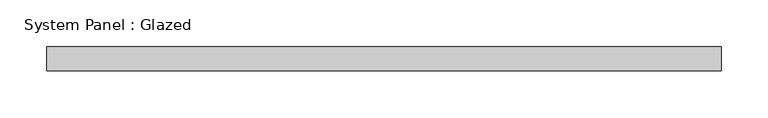
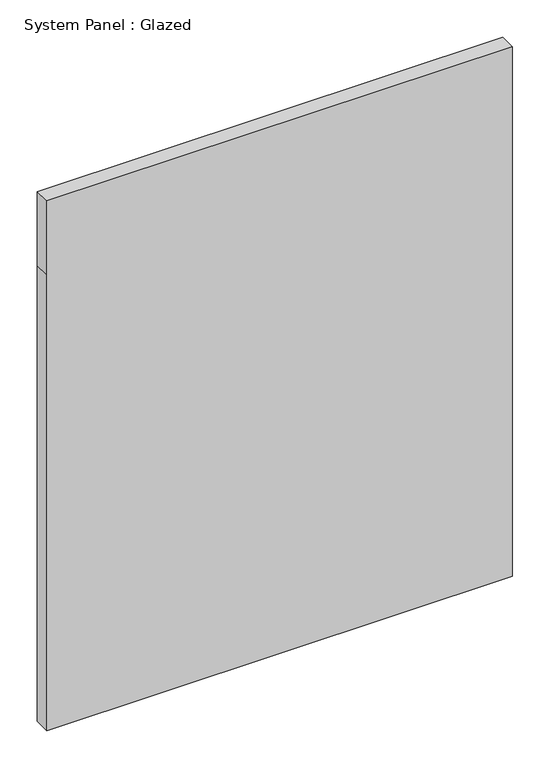
"""IFC4 building model written with IfcOpenShell, lengths in millimetres: plate geometry, System Panel : Glazed."""

from ifc_helpers import new_model, si_unit, frame, origin, place, context, project, spatial, polyline, outline, extrude, source, transform, mapped, element, save


def system_panel_glazed_ddb2445b(model_context):
    return source(origin(), model_context, "Body", "SweptSolid", [
        extrude(outline(polyline([(0.0, -358.775), (0.0, 358.775), (742.6882113, 358.775), (863.3382113, 358.775), (863.3382113, -358.775), (742.6882113, -358.775), (0.0, -358.775)])), frame((0.0, 19.05, 0.0), z_axis=(0.0, 1.0, 0.0), x_axis=(0.0, 0.0, 1.0)), (0.0, 0.0, 1.0), 25.4),
    ])


if __name__ == "__main__":
    model = new_model("IFC4")
    model_context = context("Model", 3, world=origin())
    ifc_project = project(units=[si_unit("LENGTHUNIT", "METRE", prefix="MILLI")], contexts=[model_context])
    site = spatial("IfcSite", under=ifc_project)
    building = spatial("IfcBuilding", under=site)
    placement = place(None, origin())
    system_panel_glazed_shape = system_panel_glazed_ddb2445b(model_context)
    element("IfcPlate", 1, ObjectType="System Panel : Glazed", at=placement, inside=building, context=model_context, shape_type="MappedRepresentation", body=[
        mapped(system_panel_glazed_shape, transform((0.0, 0.0, 0.0), x_axis=(1.0, 0.0, 0.0), y_axis=(0.0, 1.0, 0.0), z_axis=(0.0, 0.0, 1.0))),
    ])
    save(model, "model.ifc")

# Revit data of these elements
# Type "System Panel : Glazed"
#   Construction Type Id = "GSP4R"
#   Analytic Construction = "1/8 in Pilkington single glazing"
#   Visual Light Transmittance = 0.9
#   Solar Heat Gain Coefficient = 0.86
#   Heat Transfer Coefficient (U) = 1.18115 BTU/(h·ft²·°F)
#   Define Thermal Properties by = 1
# Element 1 (IfcPlate, "System Panel : Glazed")
#   Materials on its faces: "Glass"
# Materials
#   "Glass": class "Glass", colour RGB 0 128 192, transparency 0.75, Description = "Soda Lime Glass", Cost = 0
